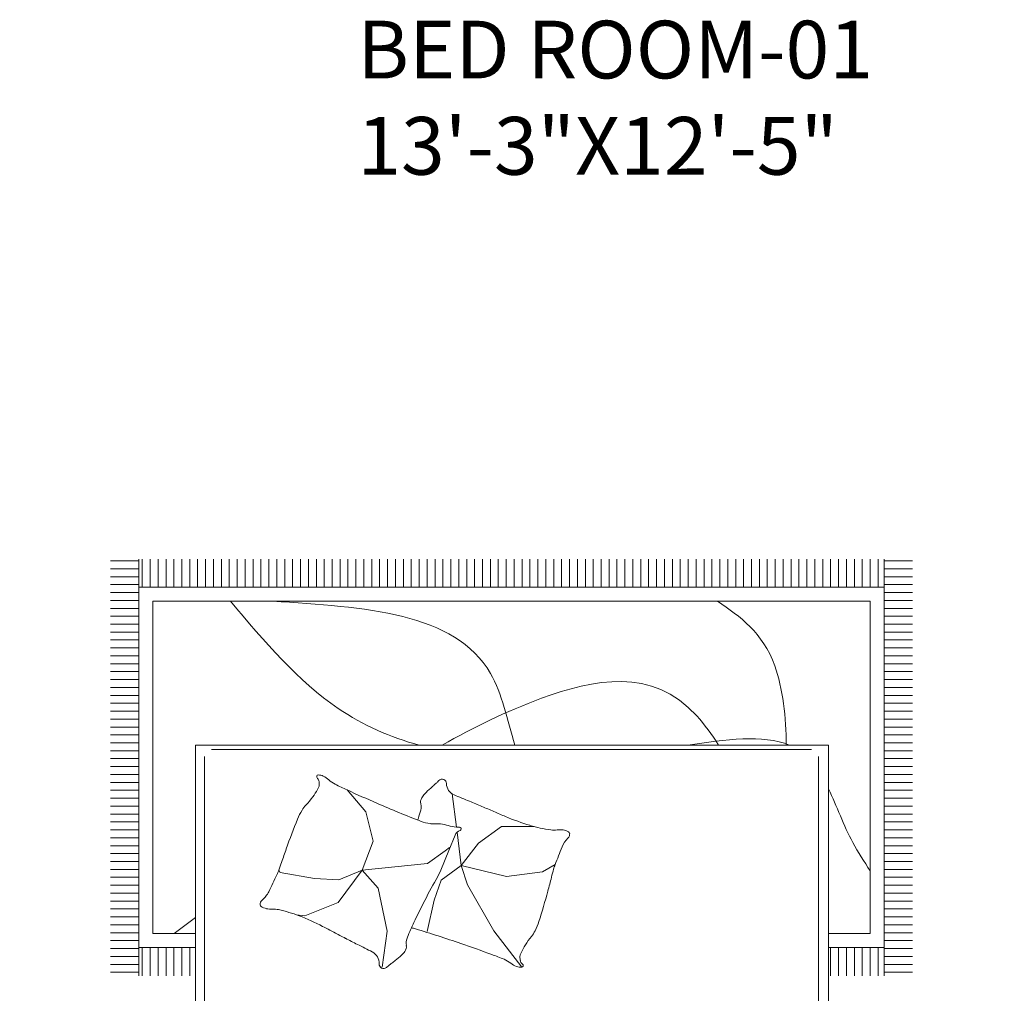
# Model space of a CAD drawing. Units: inches. Extents: x -7 to 1228, y -146 to 1091.
# Tile 68 of 88: x 657 to 743, y 617 to 702. Entities that reach past the tile are written whole.
import ezdxf

# ---------------------------------------------------------------- set-up
doc = ezdxf.new("R2010")
doc.units = ezdxf.units.IN
doc.layers.add('A-AREA-IDEN', color=7, linetype='Continuous', lineweight=18)
doc.layers.add('A-FURN', color=8, linetype='Continuous', lineweight=18)
doc.styles.add('DIM_FONT', font='SIMPLEX.shx', dxfattribs={"width": 0.8})
doc.styles.get("Standard").update_dxf_attribs({"font": 'arial.ttf'})

# ---------------------------------------------------------------- blocks, each defined once
blk = doc.blocks.new('A$C4F634EDD')
for p, q in [((0, 2.6295), (0, 2.2295)), ((0.5, 2.6295), (0, 2.6295)), ((0.5, 2.6295), (2.3, 2.6295)), ((0.5, 0.5295), (0.5, 2.6295)), ((0.5, 2.2295), (0.5, 2.6295)), ((2.3, 2.6295), (2.3, 0.5295)), ((2.3, 2.6295), (2.8, 2.6295)), ((2.3, 2.2295), (2.3, 2.6295)), ((2.8, 2.6295), (2.8, 2.2295)), ((0.5, 2.5771), (2.3, 2.5771)), ((2.392, 2.5115), (2.5692, 2.5765)), ((2.5692, 2.5765), (2.574, 2.5743)), ((0.2457, 2.5697), (0.2457, 2.4733)), ((2.4985, 2.5445), (2.5516, 2.564)), ((2.5062, 2.5454), (2.5487, 2.561)), ((2.5483, 2.5347), (2.5487, 2.561)), ((2.5487, 2.561), (2.5571, 2.56)), ((2.5615, 2.5536), (2.5514, 2.5318)), ((2.5516, 2.564), (2.5637, 2.5584)), ((2.5571, 2.56), (2.5615, 2.5536)), ((2.5615, 2.5536), (2.5791, 2.5058)), ((2.5637, 2.5584), (2.6418, 2.3458)), ((2.574, 2.5743), (2.6638, 2.3298)), ((2.4842, 2.5232), (2.47, 2.518)), ((2.4862, 2.5179), (2.4842, 2.5232)), ((2.4946, 2.5331), (2.4985, 2.5445)), ((2.5734, 2.3187), (2.4946, 2.5331)), ((2.5062, 2.5454), (2.5004, 2.5392)), ((2.5004, 2.5392), (2.5013, 2.5315)), ((2.5013, 2.5315), (2.5188, 2.4836)), ((2.5013, 2.5315), (2.5231, 2.5214)), ((2.5235, 2.5256), (2.5062, 2.5454)), ((2.5231, 2.5214), (2.5235, 2.5256)), ((2.5523, 2.4417), (2.5231, 2.5214)), ((2.5483, 2.5347), (2.5235, 2.5256)), ((2.5514, 2.5318), (2.5483, 2.5347)), ((2.5807, 2.4521), (2.5514, 2.5318)), ((2.3898, 2.5066), (2.392, 2.5115)), ((2.4795, 2.2621), (2.3898, 2.5066)), ((2.412, 2.5007), (2.4634, 2.5196)), ((2.4361, 2.4352), (2.412, 2.5007)), ((2.4634, 2.5196), (2.4875, 2.454)), ((2.47, 2.518), (2.472, 2.5127)), ((2.472, 2.5127), (2.4862, 2.5179)), ((2.4881, 2.5126), (2.4739, 2.5074)), ((2.4739, 2.5074), (2.4759, 2.502)), ((2.4759, 2.502), (2.4901, 2.5073)), ((2.492, 2.5019), (2.4778, 2.4967)), ((2.4778, 2.4967), (2.4798, 2.4914)), ((2.4798, 2.4914), (2.494, 2.4966)), ((2.4901, 2.5073), (2.4881, 2.5126)), ((2.494, 2.4966), (2.492, 2.5019)), ((2.5788, 2.4956), (2.5767, 2.4848)), ((2.5791, 2.5058), (2.5788, 2.4956)), ((2.4959, 2.4913), (2.4817, 2.4861)), ((2.4817, 2.4861), (2.4837, 2.4808)), ((2.4837, 2.4808), (2.4979, 2.486)), ((2.4998, 2.4807), (2.4856, 2.4755)), ((2.4856, 2.4755), (2.4876, 2.4702)), ((2.4876, 2.4702), (2.5018, 2.4754)), ((2.5037, 2.47), (2.4895, 2.4648)), ((2.4895, 2.4648), (2.4915, 2.4595)), ((2.4915, 2.4595), (2.5057, 2.4647)), ((2.4979, 2.486), (2.4959, 2.4913)), ((2.5018, 2.4754), (2.4998, 2.4807)), ((2.5057, 2.4647), (2.5037, 2.47)), ((2.5188, 2.4836), (2.5256, 2.4761)), ((2.5256, 2.4761), (2.5342, 2.4692)), ((2.5342, 2.4692), (2.5405, 2.4574)), ((2.5767, 2.4848), (2.5795, 2.4717)), ((2.5795, 2.4717), (2.586, 2.454)), ((2.4875, 2.454), (2.4361, 2.4352)), ((2.5405, 2.4574), (2.547, 2.4397)), ((2.5594, 2.4061), (2.547, 2.4397)), ((2.5523, 2.4417), (2.5875, 2.346)), ((2.5807, 2.4521), (2.6158, 2.3564)), ((2.5984, 2.4204), (2.586, 2.454)), ((0.0957, 2.4197), (0.192, 2.4197)), ((0.2994, 2.4197), (0.3957, 2.4197)), ((2.4457, 2.4146), (2.4563, 2.4185)), ((2.4496, 2.4039), (2.4457, 2.4146)), ((2.4563, 2.4185), (2.4602, 2.4078)), ((2.4634, 2.4211), (2.474, 2.425)), ((2.4673, 2.4104), (2.4634, 2.4211)), ((2.4779, 2.4143), (2.4673, 2.4104)), ((2.474, 2.425), (2.4779, 2.4143)), ((2.4811, 2.4276), (2.4917, 2.4315)), ((2.485, 2.4169), (2.4811, 2.4276)), ((2.4956, 2.4208), (2.485, 2.4169)), ((2.4883, 2.4081), (2.4989, 2.412)), ((2.4922, 2.3975), (2.4883, 2.4081)), ((2.4917, 2.4315), (2.4956, 2.4208)), ((2.4989, 2.412), (2.5028, 2.4014)), ((2.6047, 2.4086), (2.5984, 2.4204)), ((2.6133, 2.4017), (2.6047, 2.4086)), ((2.4602, 2.4078), (2.4496, 2.4039)), ((2.4528, 2.3951), (2.4635, 2.399)), ((2.4567, 2.3844), (2.4528, 2.3951)), ((2.4674, 2.3883), (2.4567, 2.3844)), ((2.4635, 2.399), (2.4674, 2.3883)), ((2.4706, 2.4016), (2.4812, 2.4055)), ((2.4745, 2.3909), (2.4706, 2.4016)), ((2.4851, 2.3949), (2.4745, 2.3909)), ((2.4777, 2.3821), (2.4883, 2.386)), ((2.4816, 2.3715), (2.4777, 2.3821)), ((2.4812, 2.4055), (2.4851, 2.3949)), ((2.4883, 2.386), (2.4922, 2.3754)), ((2.5028, 2.4014), (2.4922, 2.3975)), ((2.4954, 2.3886), (2.5061, 2.3925)), ((2.4993, 2.378), (2.4954, 2.3886)), ((2.51, 2.3819), (2.4993, 2.378)), ((2.5061, 2.3925), (2.51, 2.3819)), ((2.5238, 2.3769), (2.538, 2.3821)), ((2.538, 2.3821), (2.5419, 2.3715)), ((2.5622, 2.393), (2.5594, 2.4061)), ((2.5598, 2.372), (2.5601, 2.3822)), ((2.5601, 2.3822), (2.5622, 2.393)), ((2.6201, 2.3941), (2.6133, 2.4017)), ((2.6376, 2.3463), (2.6201, 2.3941)), ((2.6499, 2.3979), (2.6397, 2.3953)), ((2.6417, 2.39), (2.6488, 2.391)), ((2.6488, 2.391), (2.6538, 2.3895)), ((2.6551, 2.397), (2.6499, 2.3979)), ((2.6538, 2.3895), (2.6596, 2.388)), ((2.6627, 2.392), (2.6551, 2.397)), ((2.6596, 2.388), (2.6626, 2.3867)), ((2.6626, 2.3867), (2.6662, 2.388)), ((2.6692, 2.394), (2.6627, 2.392)), ((2.6662, 2.388), (2.6632, 2.3828)), ((2.6632, 2.3828), (2.6736, 2.3744)), ((2.6736, 2.3944), (2.6692, 2.394)), ((2.6765, 2.391), (2.6736, 2.3944)), ((2.6742, 2.3795), (2.6765, 2.391)), ((2.6824, 2.3858), (2.6742, 2.3795)), ((2.6873, 2.3815), (2.6824, 2.3858)), ((2.6853, 2.369), (2.6873, 2.3815)), ((0.2457, 2.366), (0.2457, 2.2697)), ((2.46, 2.3756), (2.4706, 2.3795)), ((2.4639, 2.365), (2.46, 2.3756)), ((2.4745, 2.3689), (2.4639, 2.365)), ((2.4672, 2.3561), (2.4778, 2.36)), ((2.4711, 2.3455), (2.4672, 2.3561)), ((2.4706, 2.3795), (2.4745, 2.3689)), ((2.4778, 2.36), (2.4817, 2.3494)), ((2.4922, 2.3754), (2.4816, 2.3715)), ((2.4849, 2.3626), (2.4955, 2.3665)), ((2.4888, 2.352), (2.4849, 2.3626)), ((2.4994, 2.3559), (2.4888, 2.352)), ((2.4955, 2.3665), (2.4994, 2.3559)), ((2.5026, 2.3691), (2.5132, 2.373)), ((2.5065, 2.3585), (2.5026, 2.3691)), ((2.5171, 2.3624), (2.5065, 2.3585)), ((2.5132, 2.373), (2.5171, 2.3624)), ((2.5277, 2.3663), (2.5238, 2.3769)), ((2.5419, 2.3715), (2.5277, 2.3663)), ((2.5774, 2.3242), (2.5598, 2.372)), ((2.6154, 2.3522), (2.5905, 2.3431)), ((2.6158, 2.3564), (2.6154, 2.3522)), ((2.6154, 2.3522), (2.6327, 2.3324)), ((2.6376, 2.3463), (2.6158, 2.3564)), ((2.6736, 2.3744), (2.6922, 2.3593)), ((2.6946, 2.376), (2.6853, 2.369)), ((2.6922, 2.3593), (2.7051, 2.3473)), ((2.6995, 2.3713), (2.6946, 2.376)), ((2.695, 2.3603), (2.6995, 2.3713)), ((2.7031, 2.3682), (2.695, 2.3603)), ((2.7096, 2.3616), (2.7031, 2.3682)), ((2.7062, 2.351), (2.7096, 2.3616)), ((2.7147, 2.3578), (2.7062, 2.351)), ((2.7214, 2.3517), (2.7147, 2.3578)), ((0, 2.3301), (0.5, 2.3301)), ((2.8, 2.3301), (2.3, 2.3301)), ((2.4817, 2.3494), (2.4711, 2.3455)), ((2.5774, 2.3242), (2.5875, 2.346)), ((2.5818, 2.3178), (2.5774, 2.3242)), ((2.5875, 2.346), (2.5905, 2.3431)), ((2.5905, 2.3431), (2.5901, 2.3168)), ((2.5901, 2.3168), (2.6097, 2.324)), ((2.613, 2.3312), (2.6077, 2.3293)), ((2.6077, 2.3293), (2.6135, 2.3141)), ((2.6192, 2.3174), (2.613, 2.3312)), ((2.6153, 2.3261), (2.6327, 2.3324)), ((2.6369, 2.332), (2.6161, 2.3243)), ((2.6616, 2.3249), (2.6234, 2.3109)), ((2.6327, 2.3324), (2.6385, 2.3386)), ((2.6418, 2.3458), (2.6369, 2.332)), ((2.6385, 2.3386), (2.6376, 2.3463)), ((2.6638, 2.3298), (2.6616, 2.3249)), ((2.7051, 2.3473), (2.7079, 2.3475)), ((2.7079, 2.3475), (2.7079, 2.3443)), ((2.7079, 2.3443), (2.727, 2.3277)), ((2.7196, 2.34), (2.7214, 2.3517)), ((2.7286, 2.3466), (2.7196, 2.34)), ((2.727, 2.3277), (2.7512, 2.2983)), ((2.7346, 2.3423), (2.7286, 2.3466)), ((2.732, 2.3295), (2.7346, 2.3423)), ((2.7423, 2.3345), (2.732, 2.3295)), ((2.7406, 2.3172), (2.7495, 2.325)), ((2.7495, 2.325), (2.7423, 2.3345)), ((2.6172, 2.3086), (2.4844, 2.2599)), ((2.5362, 2.305), (2.5185, 2.2985)), ((2.5185, 2.2985), (2.5224, 2.2879)), ((2.5401, 2.2944), (2.5362, 2.305)), ((2.561, 2.3141), (2.5433, 2.3076)), ((2.5433, 2.3076), (2.5472, 2.297)), ((2.5472, 2.297), (2.5649, 2.3035)), ((2.5649, 2.3035), (2.561, 2.3141)), ((2.5855, 2.3131), (2.5734, 2.3187)), ((2.5901, 2.3168), (2.5818, 2.3178)), ((2.6104, 2.3222), (2.5855, 2.3131)), ((2.6135, 2.3141), (2.6244, 2.2977)), ((2.626, 2.3069), (2.6192, 2.3174)), ((2.6244, 2.2977), (2.6349, 2.2825)), ((2.6365, 2.2916), (2.626, 2.3069)), ((2.7519, 2.3218), (2.7406, 2.3172)), ((2.7512, 2.2983), (2.756, 2.2695)), ((2.7575, 2.3144), (2.7519, 2.3218)), ((2.7526, 2.3045), (2.7575, 2.3144)), ((2.7622, 2.308), (2.7526, 2.3045)), ((2.7574, 2.2924), (2.7673, 2.2997)), ((2.7673, 2.2997), (2.7622, 2.308)), ((0.5953, 2.1912), (0.616, 2.2738)), ((1.4546, 2.1912), (1.4752, 2.2738)), ((2.5114, 2.2959), (2.4936, 2.2894)), ((2.4936, 2.2894), (2.4976, 2.2788)), ((2.4976, 2.2788), (2.5153, 2.2853)), ((2.5153, 2.2853), (2.5114, 2.2959)), ((2.5224, 2.2879), (2.5401, 2.2944)), ((2.6349, 2.2825), (2.638, 2.273)), ((2.6407, 2.2834), (2.6365, 2.2916)), ((2.6399, 2.2712), (2.6374, 2.2659)), ((2.638, 2.273), (2.6399, 2.2712)), ((2.6438, 2.2739), (2.6407, 2.2834)), ((2.6519, 2.2716), (2.6438, 2.2739)), ((2.6535, 2.2628), (2.6519, 2.2716)), ((2.756, 2.2695), (2.7459, 2.2483)), ((2.7687, 2.2905), (2.7574, 2.2924)), ((2.7587, 2.279), (2.7699, 2.2828)), ((2.7708, 2.2725), (2.7587, 2.279)), ((2.7699, 2.2828), (2.7687, 2.2905)), ((2.7706, 2.2643), (2.7708, 2.2725)), ((2.4844, 2.2599), (2.4795, 2.2621)), ((2.6374, 2.2659), (2.6398, 2.257)), ((2.6398, 2.257), (2.6509, 2.259)), ((2.6509, 2.259), (2.6431, 2.2492)), ((2.6431, 2.2492), (2.6473, 2.2398)), ((2.6473, 2.2398), (2.6592, 2.2429)), ((2.6592, 2.2429), (2.6521, 2.2314)), ((2.6636, 2.2409), (2.6535, 2.2628)), ((2.6836, 2.2287), (2.6636, 2.2409)), ((2.7459, 2.2483), (2.7284, 2.2317)), ((2.7509, 2.2314), (2.7459, 2.2418)), ((2.7459, 2.2418), (2.7568, 2.2352)), ((2.7529, 2.2505), (2.7645, 2.2498)), ((2.7607, 2.2424), (2.7529, 2.2505)), ((2.7568, 2.2352), (2.7607, 2.2424)), ((2.759, 2.2637), (2.7706, 2.2643)), ((2.7676, 2.2559), (2.759, 2.2637)), ((2.7645, 2.2498), (2.7676, 2.2559)), ((0, 2.2295), (0.5, 2.2295)), ((2.8, 2.2295), (2.3, 2.2295)), ((2.6521, 2.2314), (2.6598, 2.2248)), ((2.6598, 2.2248), (2.6697, 2.2309)), ((2.6697, 2.2309), (2.6684, 2.219)), ((2.6684, 2.219), (2.6761, 2.2145)), ((2.6761, 2.2145), (2.6821, 2.2237)), ((2.6821, 2.2237), (2.6843, 2.2135)), ((2.7063, 2.2256), (2.6836, 2.2287)), ((2.6843, 2.2135), (2.6927, 2.2117)), ((2.6927, 2.2117), (2.6986, 2.222)), ((2.6986, 2.222), (2.7019, 2.2098)), ((2.7284, 2.2317), (2.7063, 2.2256)), ((2.7102, 2.2104), (2.7113, 2.2218)), ((2.7113, 2.2218), (2.7192, 2.2137)), ((2.7192, 2.2137), (2.7255, 2.2152)), ((2.7255, 2.2152), (2.7242, 2.2265)), ((2.7242, 2.2265), (2.7324, 2.2165)), ((2.7324, 2.2165), (2.7386, 2.2208)), ((2.7386, 2.2208), (2.7354, 2.2306)), ((2.7354, 2.2306), (2.7462, 2.2264)), ((2.7462, 2.2264), (2.7509, 2.2314)), ((0.5878, 2.1612), (0.5953, 2.1912)), ((1.4471, 2.1612), (1.4546, 2.1912)), ((2.7019, 2.2098), (2.7102, 2.2104)), ((1.5035, 2.141), (0.5458, 2.141)), ((1.5035, 2.141), (2.2716, 1.7136)), ((0.5258, 2.121), (0.5258, 0.5617)), ((1.576, 1.9433), (1.5624, 1.8479)), ((0.5458, 1.8684), (1.5653, 1.8684)), ((1.5624, 1.8479), (1.5641, 1.7178)), ((2.2716, 0.5617), (2.2716, 1.7136)), ((0.3386, 0), (0.3386, 1.1852)), ((0.3486, 1.1052), (0.3486, 1.1852)), ((0.3711, 1.1052), (0.3711, 1.1852)), ((0.3936, 1.1052), (0.3936, 1.1852)), ((0.4161, 1.1052), (0.4161, 1.1852)), ((0.4386, 1.1052), (0.4386, 1.1852)), ((0.4611, 1.1052), (0.4611, 1.1852)), ((0.4836, 1.1052), (0.4836, 1.1852)), ((2.3061, 1.1052), (2.3061, 1.1852)), ((2.3286, 1.1052), (2.3286, 1.1852)), ((2.3511, 1.1052), (2.3511, 1.1852)), ((2.3736, 1.1052), (2.3736, 1.1852)), ((2.3961, 1.1052), (2.3961, 1.1852)), ((2.4186, 1.1052), (2.4186, 1.1852)), ((2.4411, 1.1052), (2.4411, 1.1852)), ((2.4588, 1.1852), (2.4588, 0)), ((0.2586, 1.1753), (0.3386, 1.1753)), ((0.2586, 1.1528), (0.3386, 1.1528)), ((1.031, 1.1612), (1.0448, 1.0581)), ((1.4276, 1.1611), (1.3484, 1.0571)), ((2.4588, 1.1753), (2.5388, 1.1753)), ((2.4588, 1.1528), (2.5388, 1.1528)), ((0.2586, 1.1303), (0.3386, 1.1303)), ((2.4588, 1.1303), (2.5388, 1.1303)), ((0.2586, 1.1078), (0.3386, 1.1078)), ((0.3386, 1.1052), (0.5, 1.1052)), ((2.3, 1.1052), (2.4588, 1.1052)), ((2.4588, 1.1078), (2.5388, 1.1078)), ((0.2586, 1.0853), (0.3386, 1.0853)), ((0.3786, 1.0652), (0.5, 1.0652)), ((0.3786, 0.12), (0.3786, 1.0652)), ((2.3, 1.0652), (2.4188, 1.0652)), ((2.4188, 1.0652), (2.4188, 0.12)), ((2.4588, 1.0853), (2.5388, 1.0853)), ((0.2586, 1.0628), (0.3386, 1.0628)), ((0.2586, 1.0403), (0.3386, 1.0403)), ((1.0448, 1.0581), (1.019, 0.936)), ((1.1784, 0.9702), (1.1586, 1.0591)), ((1.3484, 1.0571), (1.2733, 0.9268)), ((2.4588, 1.0628), (2.5388, 1.0628)), ((2.4588, 1.0403), (2.5388, 1.0403)), ((0.2586, 1.0178), (0.3386, 1.0178)), ((0.8108, 1.0151), (0.7868, 1.0117)), ((0.9054, 0.9773), (0.8108, 1.0151)), ((2.4588, 1.0178), (2.5388, 1.0178)), ((0.2586, 0.9953), (0.3386, 0.9953)), ((2.4588, 0.9953), (2.5388, 0.9953)), ((0.2586, 0.9728), (0.3386, 0.9728)), ((0.9743, 0.8845), (0.9054, 0.9773)), ((1.1982, 0.9129), (1.1784, 0.9702)), ((2.4588, 0.9728), (2.5388, 0.9728)), ((0.2586, 0.9503), (0.3386, 0.9503)), ((0.2586, 0.9278), (0.3386, 0.9278)), ((1.019, 0.936), (0.9743, 0.8845)), ((1.2733, 0.9268), (1.2555, 0.8715)), ((2.4588, 0.9503), (2.5388, 0.9503)), ((2.4588, 0.9278), (2.5388, 0.9278)), ((0.2586, 0.9053), (0.3386, 0.9053)), ((0.8384, 0.9085), (0.7403, 0.8913)), ((0.9072, 0.912), (0.8384, 0.9085)), ((0.9743, 0.8845), (0.9072, 0.912)), ((1.2555, 0.8715), (1.1982, 0.9129)), ((1.2555, 0.8715), (1.384, 0.9031)), ((1.384, 0.9031), (1.4868, 0.8892)), ((2.4588, 0.9053), (2.5388, 0.9053)), ((0.2586, 0.8828), (0.3386, 0.8828)), ((0.7403, 0.8913), (0.737, 0.8849)), ((0.9743, 0.8845), (1.0052, 0.802)), ((0.9743, 0.8845), (1.16, 0.8656)), ((1.1973, 0.8853), (1.2203, 0.829)), ((1.2555, 0.8715), (1.2437, 0.7773)), ((1.2555, 0.8715), (1.3049, 0.8082)), ((1.4868, 0.8892), (1.5228, 0.8692)), ((2.4588, 0.8828), (2.5388, 0.8828)), ((0.2586, 0.8603), (0.3386, 0.8603)), ((1.16, 0.8656), (1.2099, 0.8295)), ((2.4588, 0.8603), (2.5388, 0.8603)), ((0.2586, 0.8378), (0.3386, 0.8378)), ((0.2586, 0.8153), (0.3386, 0.8153)), ((1.2099, 0.8295), (1.222, 0.8209)), ((1.2203, 0.829), (1.2381, 0.7855)), ((2.4588, 0.8378), (2.5388, 0.8378)), ((2.4588, 0.8153), (2.5388, 0.8153)), ((0.2586, 0.7928), (0.3386, 0.7928)), ((1.0052, 0.802), (0.9846, 0.7194)), ((1.3049, 0.8082), (1.3701, 0.7608)), ((2.4588, 0.7928), (2.5388, 0.7928)), ((0.2586, 0.7703), (0.3386, 0.7703)), ((1.2419, 0.7626), (1.23, 0.668)), ((1.3701, 0.7608), (1.463, 0.7608)), ((2.4588, 0.7703), (2.5388, 0.7703)), ((0.2586, 0.7478), (0.3386, 0.7478)), ((2.4588, 0.7478), (2.5388, 0.7478)), ((0.2586, 0.7253), (0.3386, 0.7253)), ((0.2586, 0.7028), (0.3386, 0.7028)), ((0.9846, 0.7194), (0.931, 0.6569)), ((2.4588, 0.7253), (2.5388, 0.7253)), ((2.4588, 0.7028), (2.5388, 0.7028)), ((0.2586, 0.6803), (0.3386, 0.6803)), ((2.4588, 0.6803), (2.5388, 0.6803)), ((0.2586, 0.6578), (0.3386, 0.6578)), ((2.4588, 0.6578), (2.5388, 0.6578)), ((0.2586, 0.6353), (0.3386, 0.6353)), ((2.4588, 0.6353), (2.5388, 0.6353)), ((0.2586, 0.6128), (0.3386, 0.6128)), ((0.2586, 0.5903), (0.3386, 0.5903)), ((2.4588, 0.6128), (2.5388, 0.6128)), ((2.4588, 0.5903), (2.5388, 0.5903)), ((0.2586, 0.5678), (0.3386, 0.5678)), ((2.4588, 0.5678), (2.5388, 0.5678)), ((0.2586, 0.5453), (0.3386, 0.5453)), ((0.5458, 0.5417), (2.2516, 0.5417)), ((2.4588, 0.5453), (2.5388, 0.5453)), ((0.2586, 0.5228), (0.3386, 0.5228)), ((2.3, 0.5295), (0.5, 0.5295)), ((2.4588, 0.5228), (2.5388, 0.5228)), ((0.2586, 0.5003), (0.3386, 0.5003)), ((0.2586, 0.4778), (0.3386, 0.4778)), ((2.4588, 0.5003), (2.5388, 0.5003)), ((2.4588, 0.4778), (2.5388, 0.4778)), ((0.2586, 0.4553), (0.3386, 0.4553)), ((2.4588, 0.4553), (2.5388, 0.4553)), ((0.2586, 0.4328), (0.3386, 0.4328)), ((2.4588, 0.4328), (2.5388, 0.4328)), ((0.2586, 0.4103), (0.3386, 0.4103)), ((2.4588, 0.4103), (2.5388, 0.4103)), ((0.2586, 0.3878), (0.3386, 0.3878)), ((0.2586, 0.3653), (0.3386, 0.3653)), ((2.4588, 0.3878), (2.5388, 0.3878)), ((2.4588, 0.3653), (2.5388, 0.3653)), ((0.2586, 0.3428), (0.3386, 0.3428)), ((2.4588, 0.3428), (2.5388, 0.3428)), ((0.2586, 0.3203), (0.3386, 0.3203)), ((2.4588, 0.3203), (2.5388, 0.3203)), ((0.2586, 0.2978), (0.3386, 0.2978)), ((2.4588, 0.2978), (2.5388, 0.2978)), ((0.2586, 0.2753), (0.3386, 0.2753)), ((0.2586, 0.2528), (0.3386, 0.2528)), ((2.4588, 0.2753), (2.5388, 0.2753)), ((2.4588, 0.2528), (2.5388, 0.2528)), ((0.2586, 0.2303), (0.3386, 0.2303)), ((2.4588, 0.2303), (2.5388, 0.2303)), ((0.2586, 0.2078), (0.3386, 0.2078)), ((2.4588, 0.2078), (2.5388, 0.2078)), ((0.2586, 0.1853), (0.3386, 0.1853)), ((2.4588, 0.1853), (2.5388, 0.1853)), ((0.2586, 0.1628), (0.3386, 0.1628)), ((0.2586, 0.1403), (0.3386, 0.1403)), ((2.4588, 0.1628), (2.5388, 0.1628)), ((2.4588, 0.1403), (2.5388, 0.1403)), ((0.2586, 0.1178), (0.3386, 0.1178)), ((2.4188, 0.12), (0.3786, 0.12)), ((2.4588, 0.1178), (2.5388, 0.1178)), ((0.2586, 0.0953), (0.3386, 0.0953)), ((2.4588, 0.0953), (2.5388, 0.0953)), ((0.2586, 0.0728), (0.3386, 0.0728)), ((2.4588, 0.08), (0.3386, 0.08)), ((0.3486, 0), (0.3486, 0.08)), ((0.3711, 0), (0.3711, 0.08)), ((0.3936, 0), (0.3936, 0.08)), ((0.4161, 0), (0.4161, 0.08)), ((0.4386, 0), (0.4386, 0.08)), ((0.4611, 0), (0.4611, 0.08)), ((0.4836, 0), (0.4836, 0.08)), ((0.5061, 0), (0.5061, 0.08)), ((0.5286, 0), (0.5286, 0.08)), ((0.5511, 0), (0.5511, 0.08)), ((0.5736, 0), (0.5736, 0.08)), ((0.5961, 0), (0.5961, 0.08)), ((0.6186, 0), (0.6186, 0.08)), ((0.6411, 0), (0.6411, 0.08)), ((0.6636, 0), (0.6636, 0.08)), ((0.6861, 0), (0.6861, 0.08)), ((0.7086, 0), (0.7086, 0.08)), ((0.7311, 0), (0.7311, 0.08)), ((0.7536, 0), (0.7536, 0.08)), ((0.7761, 0), (0.7761, 0.08)), ((0.7986, 0), (0.7986, 0.08)), ((0.8211, 0), (0.8211, 0.08)), ((0.8436, 0), (0.8436, 0.08)), ((0.8661, 0), (0.8661, 0.08)), ((0.8886, 0), (0.8886, 0.08)), ((0.9111, 0), (0.9111, 0.08)), ((0.9336, 0), (0.9336, 0.08)), ((0.9561, 0), (0.9561, 0.08)), ((0.9786, 0), (0.9786, 0.08)), ((1.0011, 0), (1.0011, 0.08)), ((1.0236, 0), (1.0236, 0.08)), ((1.0461, 0), (1.0461, 0.08)), ((1.0686, 0), (1.0686, 0.08)), ((1.0911, 0), (1.0911, 0.08)), ((1.1136, 0), (1.1136, 0.08)), ((1.1361, 0), (1.1361, 0.08)), ((1.1586, 0), (1.1586, 0.08)), ((1.1811, 0), (1.1811, 0.08)), ((1.2036, 0), (1.2036, 0.08)), ((1.2261, 0), (1.2261, 0.08)), ((1.2486, 0), (1.2486, 0.08)), ((1.2711, 0), (1.2711, 0.08)), ((1.2936, 0), (1.2936, 0.08)), ((1.3161, 0), (1.3161, 0.08)), ((1.3386, 0), (1.3386, 0.08)), ((1.3611, 0), (1.3611, 0.08)), ((1.3836, 0), (1.3836, 0.08)), ((1.4061, 0), (1.4061, 0.08)), ((1.4286, 0), (1.4286, 0.08)), ((1.4511, 0), (1.4511, 0.08)), ((1.4736, 0), (1.4736, 0.08)), ((1.4961, 0), (1.4961, 0.08)), ((1.5186, 0), (1.5186, 0.08)), ((1.5411, 0), (1.5411, 0.08)), ((1.5636, 0), (1.5636, 0.08)), ((1.5861, 0), (1.5861, 0.08)), ((1.6086, 0), (1.6086, 0.08)), ((1.6311, 0), (1.6311, 0.08)), ((1.6536, 0), (1.6536, 0.08)), ((1.6761, 0), (1.6761, 0.08)), ((1.6986, 0), (1.6986, 0.08)), ((1.7211, 0), (1.7211, 0.08)), ((1.7436, 0), (1.7436, 0.08)), ((1.7661, 0), (1.7661, 0.08)), ((1.7886, 0), (1.7886, 0.08)), ((1.8111, 0), (1.8111, 0.08)), ((1.8336, 0), (1.8336, 0.08)), ((1.8561, 0), (1.8561, 0.08)), ((1.8786, 0), (1.8786, 0.08)), ((1.9011, 0), (1.9011, 0.08)), ((1.9236, 0), (1.9236, 0.08)), ((1.9461, 0), (1.9461, 0.08)), ((1.9686, 0), (1.9686, 0.08)), ((1.9911, 0), (1.9911, 0.08)), ((2.0136, 0), (2.0136, 0.08)), ((2.0361, 0), (2.0361, 0.08)), ((2.0586, 0), (2.0586, 0.08)), ((2.0811, 0), (2.0811, 0.08)), ((2.1036, 0), (2.1036, 0.08)), ((2.1261, 0), (2.1261, 0.08)), ((2.1486, 0), (2.1486, 0.08)), ((2.1711, 0), (2.1711, 0.08)), ((2.1936, 0), (2.1936, 0.08)), ((2.2161, 0), (2.2161, 0.08)), ((2.2386, 0), (2.2386, 0.08)), ((2.2611, 0), (2.2611, 0.08)), ((2.2836, 0), (2.2836, 0.08)), ((2.3061, 0), (2.3061, 0.08)), ((2.3286, 0), (2.3286, 0.08)), ((2.3511, 0), (2.3511, 0.08)), ((2.3736, 0), (2.3736, 0.08)), ((2.3961, 0), (2.3961, 0.08)), ((2.4186, 0), (2.4186, 0.08)), ((2.4411, 0), (2.4411, 0.08)), ((2.4588, 0.0728), (2.5388, 0.0728)), ((0.2586, 0.0503), (0.3386, 0.0503)), ((2.4588, 0.0503), (2.5388, 0.0503)), ((0.2586, 0.0278), (0.3386, 0.0278)), ((0.2586, 0.0053), (0.3386, 0.0053)), ((2.4588, 0.0278), (2.5388, 0.0278)), ((2.4588, 0.0053), (2.5388, 0.0053))]:
    blk.add_line(p, q)
for radius in [0.1222, 0.0865]:
    blk.add_circle((0.2457, 2.4197), radius)
for centre, radius, start, end in [((0.5848, 2.5274), 0.0131, 101.2724, 206.5805), ((0.6036, 2.5368), 0.0342, 206.5805, 265.5998), ((0.5999, 2.4516), 0.0904, 90, 101.2724), ((0.5999, 2.3808), 0.1611, 81.5628, 90), ((0.5788, 2.2388), 0.3048, 74.256, 81.5628), ((0.7272, 2.7653), 0.2422, 254.256, 262.4531), ((0.7851, 3.2019), 0.6827, 262.4531, 270), ((0.7851, 3.5682), 1.049, 270, 276.0867), ((0.8402, 3.0514), 0.5293, 276.0867, 280.1899), ((1.1602, -8.1346), 10.6675, 90.30153, 91.21582), ((1.1169, 2.2433), 0.2897, 85.1982, 92.5386), ((1.2142, 3.4021), 0.8732, 265.1982, 269.4243), ((1.3082, 2.3102), 0.234, 110.8603, 117.2396), ((1.2204, 4.0232), 1.4943, 269.4243, 271.9079), ((1.2995, 2.4357), 0.0992, 105.9352, 126.0864), ((1.2429, 3.3501), 0.8208, 271.9079, 275.2592), ((1.2995, 2.4357), 0.0992, 85.7841, 105.9352), ((1.3132, 2.5864), 0.0539, 275.2592, 300.6513), ((1.3554, 2.5152), 0.0289, 85.6975, 120.6513), ((1.3556, 2.519), 0.0251, 68.2117, 85.6975), ((1.3739, 2.5288), 0.0156, 158.0096, 201.421), ((1.3634, 2.533), 0.00428, 78.1069, 158.0096), ((1.3288, 2.5111), 0.0328, 351.8665, 21.421), ((1.3647, 2.5395), 0.00232, 258.1069, 19.564), ((1.3637, 2.5391), 0.00342, 19.564, 68.2117), ((1.444, 2.5274), 0.0131, 101.2724, 206.5805), ((1.4628, 2.5368), 0.0342, 206.5805, 265.5998), ((1.4591, 2.4516), 0.0904, 90, 101.2724), ((1.4591, 2.3808), 0.1611, 81.5628, 90), ((1.438, 2.2388), 0.3048, 74.256, 81.5628), ((1.5865, 2.7653), 0.2422, 254.256, 262.4531), ((1.6443, 3.2019), 0.6827, 262.4531, 270), ((1.6443, 3.5682), 1.049, 270, 276.0867), ((1.4785, 15.4878), 12.9656, 271.22425, 272.05324), ((1.97, 2.3805), 0.1524, 92.5386, 100.1899), ((1.9761, 2.2433), 0.2897, 85.1982, 92.5386), ((2.0734, 3.4021), 0.8732, 265.1982, 269.4243), ((2.1674, 2.3102), 0.234, 110.8603, 117.2396), ((2.0797, 4.0232), 1.4943, 269.4243, 271.9079), ((2.1588, 2.4357), 0.0992, 105.9352, 126.0864), ((2.1021, 3.3501), 0.8208, 271.9079, 275.2592), ((2.1588, 2.4357), 0.0992, 85.7841, 105.9352), ((2.1724, 2.5864), 0.0539, 275.2592, 300.6513), ((2.2146, 2.5152), 0.0289, 85.6975, 120.6513), ((2.2149, 2.519), 0.0251, 68.2117, 85.6975), ((2.2331, 2.5288), 0.0156, 158.0096, 201.421), ((2.2226, 2.533), 0.00428, 78.1069, 158.0096), ((2.1881, 2.5111), 0.0328, 351.8665, 21.421), ((2.224, 2.5395), 0.00232, 258.1069, 19.564), ((2.2229, 2.5391), 0.00342, 19.564, 68.2117), ((1.0898, 2.4496), 0.4918, 173.7676, 180), ((0.5368, 2.3783), 0.1399, 45.0976, 62.7964), ((1.4317, 2.2032), 0.3916, 128.3886, 133.8115), ((1.2362, 2.45), 0.0768, 117.2396, 128.3886), ((1.2995, 2.4357), 0.0992, 143.8234, 161.5603), ((1.2995, 2.4357), 0.0992, 126.0864, 143.8234), ((1.1177, 2.5413), 0.246, 347.8905, 351.8665), ((1.949, 2.4496), 0.4918, 173.7676, 180), ((2.291, 2.2032), 0.3916, 128.3886, 133.8115), ((2.0954, 2.45), 0.0768, 117.2396, 128.3886), ((2.1588, 2.4357), 0.0992, 143.8234, 161.5603), ((2.1588, 2.4357), 0.0992, 126.0864, 143.8234), ((1.977, 2.5413), 0.246, 347.8905, 351.8665), ((0.5462, 2.4142), 0.0899, 41.4429, 53.7359), ((0.5741, 2.4389), 0.0526, 25.3551, 41.4429), ((0.5368, 2.3783), 0.1399, 27.3988, 45.0976), ((1.1799, 2.4341), 0.0493, 140.9651, 151.6832), ((1.3165, 2.3233), 0.2252, 133.8115, 140.9651), ((2.2605, 2.3525), 0.9131, 172.3191, 176.6313), ((1.5522, 2.448), 0.1983, 167.8905, 172.3191), ((2.0391, 2.4341), 0.0493, 140.9651, 151.6832), ((2.1757, 2.3233), 0.2252, 133.8115, 140.9651), ((3.1198, 2.3525), 0.9131, 172.3191, 176.6313), ((2.4114, 2.448), 0.1983, 167.8905, 172.3191), ((0.8019, 2.4496), 0.204, 180, 189.6844), ((0.4851, 2.3967), 0.1511, 21.8149, 25.3551), ((0.4345, 2.3765), 0.2056, 18.7799, 21.8149), ((0.576, 2.4246), 0.0562, 0, 18.7799), ((0.5368, 2.3783), 0.1399, 16.515, 27.3988), ((1.3127, 2.3625), 0.2002, 151.6832, 156.9972), ((1.6611, 2.4496), 0.204, 180, 189.6844), ((2.1719, 2.3625), 0.2002, 151.6832, 156.9972), ((1.4703, 2.5637), 0.882, 189.6844, 192.1984), ((0.5406, 2.4246), 0.0915, 345.3149, 0), ((0.5368, 2.3783), 0.1399, 5.6311, 16.515), ((2.3295, 2.5637), 0.882, 189.6844, 192.1984), ((2.0266, 2.3663), 0.6787, 176.6313, 181.6331), ((2.8858, 2.3663), 0.6787, 176.6313, 181.6331), ((0.2982, 2.3103), 0.3171, 8.0051, 12.1984), ((-0.0401, 2.2627), 0.6588, 2.6649, 8.0051), ((1.1575, 2.3103), 0.3171, 8.0051, 12.1984), ((0.8191, 2.2627), 0.6588, 2.6649, 8.0051), ((2.7128, 2.3859), 1.3652, 181.6331, 183.055), ((3.5721, 2.3859), 1.3652, 181.6331, 183.055), ((14.9657, 3.0398), 13.6356, 183.05496, 183.50486), ((15.8249, 3.0398), 13.6356, 183.05496, 183.50486), ((0.5503, 2.2902), 0.0677, 345.9548, 2.6649), ((1.4096, 2.2902), 0.0677, 345.9548, 2.6649), ((1.1303, 1.9835), 0.2721, 85.9172, 93.5552), ((1.1455, 2.197), 0.058, 69.3257, 85.9172), ((0.9871, 1.7772), 0.5066, 65.6735, 69.3257), ((0.473, 2.8815), 0.7387, 293.4844, 295.3111), ((0.6058, 0.9338), 1.4323, 63.5015, 65.6735), ((1.1054, 1.9358), 0.3126, 57.865, 63.5015), ((1.3322, 2.8815), 0.7387, 293.4844, 295.3111), ((0.473, 2.8815), 0.7387, 287.1982, 289.428), ((0.473, 2.8815), 0.7387, 289.428, 291.6577), ((0.473, 2.8815), 0.7387, 291.6577, 293.4844), ((0.8841, 1.5835), 0.7286, 54.1737, 57.865), ((1.6762, 2.2258), 0.3212, 183.5049, 189.9984), ((1.3322, 2.8815), 0.7387, 287.1982, 289.428), ((1.3322, 2.8815), 0.7387, 289.428, 291.6577), ((1.3322, 2.8815), 0.7387, 291.6577, 293.4844), ((2.5355, 2.2258), 0.3212, 183.5049, 189.9984), ((0.5887, 2.1609), 0.000917, 165.9551, 274.0829), ((0.5695, 2.4301), 0.2708, 274.0829, 279.4841), ((0.5763, 2.3896), 0.2297, 279.4841, 287.3864), ((0.6807, 2.0561), 0.1197, 96.4341, 107.3864), ((0.6836, 2.0301), 0.1459, 78.4414, 96.4341), ((0.759, 2.3985), 0.2301, 258.4414, 272.7491), ((0.7026, 3.5718), 1.4048, 272.7491, 274.6176), ((0.9136, 0.9591), 1.2165, 92.6096, 94.6176), ((1.2501, -19.8405), 22.0183, 90.37908, 91.01965), ((1.2012, -3.5404), 5.7185, 89.7135, 90.9704), ((1.224, 1.0141), 1.164, 86.426, 89.7135), ((1.2875, 2.0302), 0.1459, 77.131, 86.426), ((1.3099, 2.1283), 0.0453, 62.7159, 77.131), ((1.3658, 2.2367), 0.0767, 242.7159, 253.7788), ((1.3688, 2.247), 0.0875, 253.7788, 262.8796), ((1.3581, 2.1615), 0.00132, 262.8796, 343.3022), ((1.3409, 2.1667), 0.0193, 343.3022, 9.9984), ((1.448, 2.1609), 0.000917, 165.9551, 274.0829), ((1.4288, 2.4301), 0.2708, 274.0829, 279.4841), ((1.4355, 2.3896), 0.2297, 279.4841, 287.3864), ((1.5399, 2.0561), 0.1197, 96.4341, 107.3864), ((1.5429, 2.0301), 0.1459, 78.4414, 96.4341), ((1.6182, 2.3985), 0.2301, 258.4414, 272.7491), ((1.5619, 3.5718), 1.4048, 272.7491, 274.6176), ((1.7729, 0.9591), 1.2165, 92.6096, 94.6176), ((2.1093, -19.8405), 22.0183, 90.37908, 91.01965), ((2.0605, -3.5404), 5.7185, 89.7135, 90.9704), ((2.0833, 1.0141), 1.164, 86.426, 89.7135), ((2.1467, 2.0302), 0.1459, 77.131, 86.426), ((2.1691, 2.1283), 0.0453, 62.7159, 77.131), ((2.2251, 2.2367), 0.0767, 242.7159, 253.7788), ((2.2281, 2.247), 0.0875, 253.7788, 262.8796), ((2.2174, 2.1615), 0.00132, 262.8796, 343.3022), ((2.2001, 2.1667), 0.0193, 343.3022, 9.9984), ((0.5458, 2.121), 0.02, 90, 180), ((1.2147, 1.9017), 0.3751, 20.1488, 39.6445), ((1.3977, 1.9688), 0.1801, 351.8644, 20.1488), ((0.5458, 1.8884), 0.02, 180, 270), ((1.4194, 4.2174), 2.5158, 281.6741, 283.1904), ((2.0378, 1.5789), 0.1942, 97.7304, 103.1904), ((2.0195, 1.7137), 0.0581, 79.2724, 97.7304), ((1.2737, -2.2227), 4.0646, 77.0745, 79.2724), ((0.6102, 18.0525), 16.3521, 273.75703, 274.62393), ((2.0359, 1.0981), 0.6574, 74.0648, 77.0745), ((1.0582, 5.4638), 3.7801, 277.692, 279.495), ((1.7125, -0.0344), 1.8351, 72.2636, 74.0648), ((0.9863, 1.1494), 0.0359, 297.2902, 3.2455), ((1.0348, 1.1521), 0.0127, 51.1864, 183.2455), ((0.9991, 1.1077), 0.0697, 45.8726, 51.1864), ((1.0791, 1.1902), 0.0452, 225.8726, 232.4713), ((1.2846, 1.4577), 0.3825, 232.4713, 233.7837), ((0.6683, 0.6162), 0.6605, 52.7849, 53.7837), ((1.3469, 1.2115), 0.0792, 292.7069, 308.5854), ((1.4338, 1.1026), 0.0601, 110.3452, 128.5854), ((1.4251, 1.1259), 0.0352, 86.0516, 110.3452), ((1.4376, 1.1398), 0.0142, 126.5792, 169.5926), ((1.4273, 1.1567), 0.00443, 13.2808, 86.0516), ((1.4254, 1.1562), 0.0063, 306.5792, 13.2808), ((0.9362, 0.9689), 0.2176, 46.4776, 52.7849), ((1.0327, 1.0706), 0.0774, 35.8936, 46.4776), ((-0.4107, 5.9078), 5.0942, 289.0836, 290.1287), ((1.0543, 1.9106), 0.8371, 290.1287, 292.7069), ((1.4996, 1.1284), 0.0771, 169.5926, 177.2714), ((1.4378, 1.1314), 0.0153, 177.2714, 194.5709), ((1.4611, 1.1374), 0.0393, 194.5709, 206.8179), ((1.8575, -0.7096), 2.0162, 116.4147, 117.4999), ((-0.4173, 3.8699), 3.0972, 296.4147, 297.2902), ((1.0771, 1.1027), 0.0226, 351.9508, 35.8936), ((1.1449, 1.0931), 0.0458, 171.9508, 202.4162), ((0.2266, 4.0657), 3.145, 286.6085, 289.0836), ((1.7401, 1.2785), 0.352, 206.8179, 210.9056), ((1.6045, 1.1973), 0.194, 210.9056, 219.7005), ((3.744, -4.3336), 6.1019, 117.49986, 117.84822), ((2.032, 1.4591), 1.0054, 202.4162, 205.0529), ((1.3929, 1.0217), 0.081, 26.0735, 39.7005), ((0.5736, 1.5979), 0.6236, 290.7486, 297.4921), ((-1.8336, 6.2238), 5.8383, 297.49208, 297.84822), ((1.0922, 1.1636), 0.1166, 280.7366, 286.6085), ((1.2892, 0.9709), 0.1965, 17.8396, 26.0735), ((0.6422, 1.4168), 0.43, 282.6252, 290.7486), ((2.6493, 1.7476), 1.6868, 205.0529, 207.0884), ((-0.4304, 0.4175), 2.003, 15.2625, 17.8396), ((0.6894, 0.9832), 0.0058, 121.6917, 179.0386), ((0.7004, 0.983), 0.0168, 179.0386, 229.4914), ((0.7131, 0.9448), 0.0509, 103.0402, 121.6917), ((0.7152, 0.9361), 0.0599, 86.6119, 103.0402), ((0.7224, 1.0587), 0.063, 266.6119, 282.6252), ((0.6405, 0.9128), 0.0755, 26.3332, 49.4914), ((2.541, 1.6922), 1.5652, 207.0884, 209.936), ((-1.6775, -0.2344), 2.6619, 25.1732, 26.3332), ((-0.0881, 0.5109), 1.6481, 13.841, 15.2625), ((0.5689, 0.8213), 0.1798, 20.7081, 25.1732), ((0.9989, 0.8042), 0.2143, 22.2355, 29.936), ((2.0418, 1.0357), 0.5454, 193.841, 196.3122), ((0.2268, 0.692), 0.5454, 18.2369, 20.7081), ((1.6908, 0.933), 0.1798, 196.3122, 200.7773), ((4.0115, 1.8135), 2.6619, 200.7773, 201.9373), ((2.3102, 1.3785), 1.6481, 198.2369, 199.6584), ((2.6444, 1.4979), 2.003, 199.6584, 202.2355), ((1.6124, 0.8472), 0.0755, 201.9373, 225.0955), ((1.2594, 0.7942), 0.0231, 202.2355, 252.8133), ((1.5473, 0.7819), 0.0168, 354.6428, 45.0955), ((1.1727, 0.9313), 0.1794, 277.6784, 284.8807), ((1.2689, 0.569), 0.1955, 97.9822, 104.8807), ((1.2465, 0.729), 0.034, 85.7407, 97.9822), ((1.2497, 0.772), 0.0092, 265.7407, 289.3799), ((1.2512, 0.7678), 0.00467, 289.3799, 72.8133), ((1.6266, 0.159), 0.6236, 106.3527, 113.0962), ((1.5721, 0.3449), 0.43, 98.2293, 106.3527), ((1.5195, 0.708), 0.063, 82.216, 98.2293), ((1.5362, 0.8298), 0.0599, 262.216, 278.6443), ((1.5375, 0.8209), 0.0509, 278.6443, 297.2959), ((1.5582, 0.7808), 0.0058, 297.2959, 354.6428), ((0.9722, 0.8143), 0.1965, 202.2355, 210.4694), ((2.2689, -2.1899), 3.145, 111.0043, 113.4795), ((0.1831, 0.4093), 1.0054, 18.0203, 19.3448), ((1.1834, 0.6373), 0.1166, 98.1216, 111.0043), ((1.1763, 0.687), 0.0663, 85.4882, 98.1216), ((1.1871, 0.8241), 0.0712, 265.4882, 277.6784), ((3.6722, -4.6377), 5.8383, 113.0962, 113.45234), ((0.8727, 0.7557), 0.081, 210.4694, 224.0964), ((1.0957, 0.7061), 0.0458, 347.5549, 18.0203), ((0.5234, 2.5582), 2.0162, 292.0188, 293.104), ((-1.0798, 6.3161), 6.1019, 293.10398, 293.45234), ((0.6752, 0.5644), 0.194, 35.3015, 44.0964), ((0.5462, 0.4731), 0.352, 31.2138, 35.3015), ((3.0455, -3.9778), 5.0942, 113.4795, 114.5246), ((1.1625, 0.6914), 0.0226, 167.5549, 211.4977), ((1.2092, 0.72), 0.0774, 211.4977, 222.0817), ((2.4404, -2.1823), 3.0972, 112.0188, 112.8944), ((0.8136, 0.6351), 0.0393, 18.9668, 31.2138), ((0.8364, 0.6429), 0.0153, 1.6673, 18.9668), ((1.2784, -0.1047), 0.8371, 114.5246, 117.1028), ((1.3133, 0.814), 0.2176, 222.0817, 228.389), ((1.6074, 1.1451), 0.6605, 228.389, 229.3878), ((1.2495, 0.6379), 0.0359, 112.8944, 178.8496), ((0.8506, 0.6191), 0.0063, 130.9751, 197.6767), ((0.8488, 0.6185), 0.00443, 197.6767, 270.4475), ((0.8372, 0.6345), 0.0142, 310.9751, 353.9885), ((0.8486, 0.6493), 0.0352, 270.4475, 294.7411), ((0.7746, 0.6411), 0.0771, 353.9885, 1.6673), ((0.8382, 0.6719), 0.0601, 294.7411, 312.9813), ((0.9332, 0.57), 0.0792, 117.1028, 132.9813), ((0.9284, 0.3533), 0.3825, 48.0754, 49.3878), ((1.1538, 0.6043), 0.0452, 41.4767, 48.0754), ((1.2399, 0.6804), 0.0697, 221.4767, 226.7905), ((1.2009, 0.6389), 0.0127, 226.7905, 358.8496)]:
    blk.add_arc(centre, radius, start, end)
for points in [[(0.4393, 1.0652), (0.4595, 1.05), (0.4798, 1.0348), (0.5, 1.0195)], [(1.9003, 0.5295), (2.0065, 0.514), (2.1132, 0.4978), (2.1894, 0.5295)]]:
    blk.add_open_spline(points, degree=3)
for points, knots in [([(2.3, 0.6535), (2.3236, 0.7026), (2.3554, 0.7914), (2.4015, 0.8608), (2.4188, 0.8868)], [1893.525221, 1893.525221, 1893.525221, 1893.525221, 2051.902476, 2146.74457, 2146.74457, 2146.74457, 2146.74457]), ([(0.5992, 0.12), (0.6957, 0.2341), (0.8523, 0.4189), (1.0536, 0.5069), (1.136, 0.5295)], [0, 0, 0, 0, 432.822832, 701.445452, 701.445452, 701.445452, 701.445452]), ([(0.7187, 0.12), (0.9791, 0.1362), (1.326, 0.1577), (1.3868, 0.4574), (1.408, 0.5295)], [0, 0, 0, 0, 653.160442, 870.050857, 870.050857, 870.050857, 870.050857]), ([(1.2016, 0.5295), (1.2892, 0.479), (1.5144, 0.3684), (1.8265, 0.2994), (1.9681, 0.4992), (1.9875, 0.5295)], [936.534237, 936.534237, 936.534237, 936.534237, 1243.285375, 1683.261222, 1758.254386, 1758.254386, 1758.254386, 1758.254386]), ([(2.1796, 0.5295), (2.1798, 0.4519), (2.1548, 0.2369), (2.0487, 0.164), (1.9846, 0.12)], [2202.034493, 2202.034493, 2202.034493, 2202.034493, 2357.807635, 2594.446174, 2594.446174, 2594.446174, 2594.446174])]:
    blk.add_open_spline(points, degree=3, knots=knots)
at = {"style": 'DIM_FONT', "width": 0.8, "flags": 9}
for tag, p in [('YSIZE', (0.5, 2.6295)), ('XSIZE', (0.5, 2.6295)), ('XSIZE', (2.2985, 2.6295)), ('YSIZE', (2.2985, 2.6295))]:
    blk.add_attdef(tag, p, '', height=0.0005, dxfattribs=at)

msp = doc.modelspace()

# ---------------------------------------------------------------- block references
at = {"layer": 'A-FURN', "xscale": -30.79356024027943, "yscale": 30.79356024027943, "zscale": 30.79356024027943, "rotation": 180}
msp.add_blockref('A$C4F634EDD', (656.965, 654.972), dxfattribs=at)

# ---------------------------------------------------------------- texts
at = {"layer": 'A-AREA-IDEN', "insert": (686.527, 702.116), "char_height": 5.05676, "attachment_point": 1}
msp.add_mtext_dynamic_manual_height_columns('BED ROOM-01\\P13\'-3"X12\'-5"', width=137.28212, gutter_width=25.284, heights=[0], dxfattribs=at)

doc.saveas('drawing.dxf')
